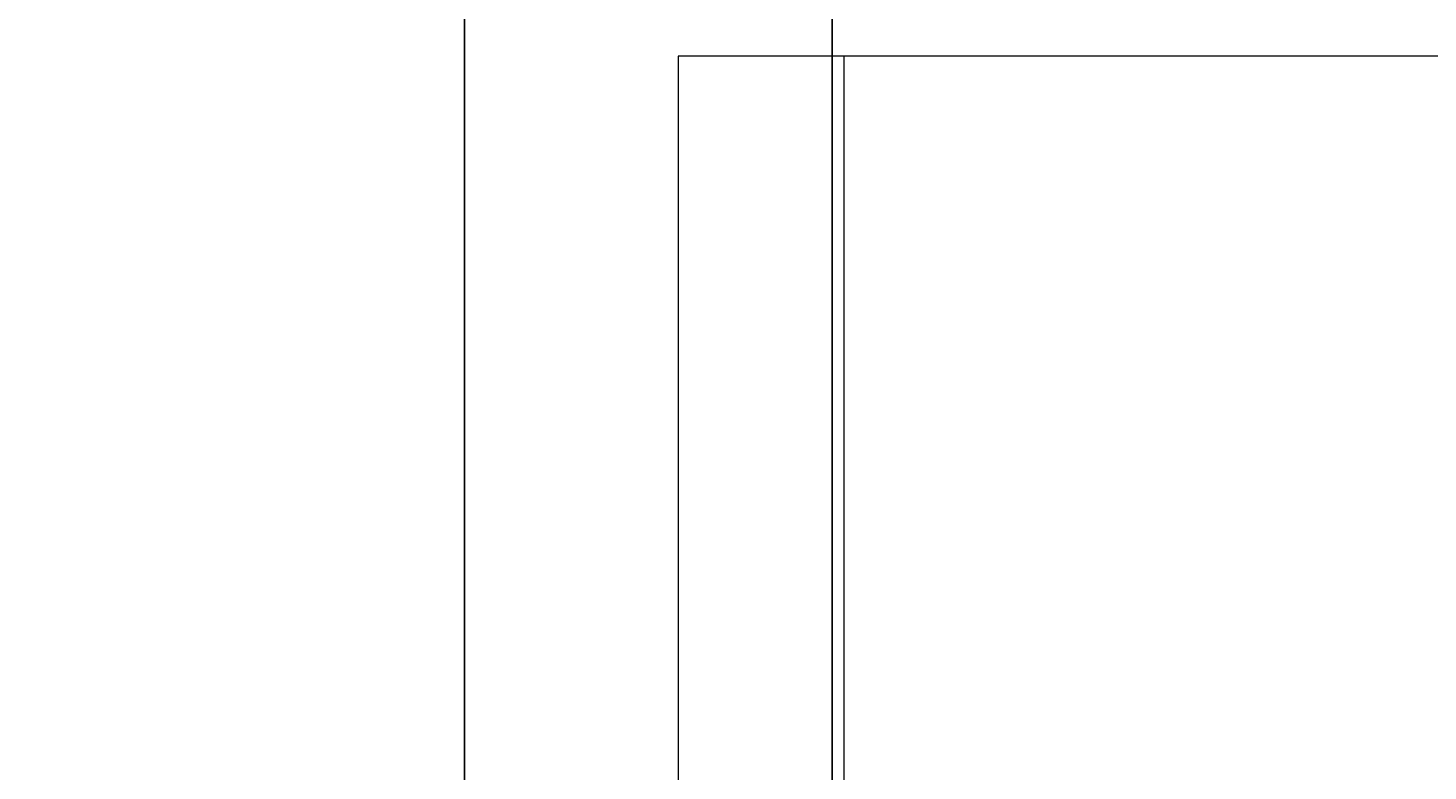
# Model space of a CAD drawing. Units: inches. Extents: x 1998 to 2588, y 1139 to 1977.
# Tile 124 of 134: x 2398 to 2429, y 1653 to 1669. Entities that reach past the tile are written whole.
import ezdxf

# ---------------------------------------------------------------- set-up
doc = ezdxf.new("R2010")
doc.units = ezdxf.units.IN
doc.layers.add('A-ANNO-DIMS', color=2, linetype='Continuous', lineweight=18)
doc.layers.add('FUR', color=21, linetype='Continuous', lineweight=18)
doc.styles.get("Standard").update_dxf_attribs({"font": 'arial.ttf'})
doc.dimstyles.get("Standard").update_dxf_attribs({"dimtxt": 0.18, "dimasz": 0.18, "dimexe": 0.18, "dimexo": 0.0625, "dimgap": 0.09, "dimtad": 0, "dimtih": 1, "dimtoh": 1, "dimdec": 4, "dimzin": 0, "dimdsep": 46, "dimtxsty": 'Standard', "dimcen": 0.09, "dimadec": 0, "dimazin": 0, "dimtfac": 1, "dimtdec": 4, "dimtofl": 0, "dimtmove": 0, "dimatfit": 3, "dimfxl": 1, "dimtolj": 1, "dimtzin": 0, "dimarcsym": 0})

# ---------------------------------------------------------------- blocks, each defined once
blk = doc.blocks.new('SOFA-THREE-SEAT')
for p, q in [((3.604, 25.615), (0, 25.615)), ((0, 25.615), (0, 0))]:
    blk.add_line(p, q)
blk.add_lwpolyline([(3.604, 2.416), (71.008, 2.416), (71.008, 25.615), (3.604, 25.615)], close=True)
blk = doc.blocks.new('*D24')
at = {"layer": 'A-ANNO-DIMS', "color": 0, "lineweight": -2, "transparency": 16777216}
for p, q in [((2398.535, 1911.232), (2588.309, 1911.232)), ((2588.129, 1911.052), (2588.129, 1570.164)), ((2588.129, 1228.912), (2588.129, 1569.8)), ((2527.535, 1228.732), (2588.309, 1228.732))]:
    blk.add_line(p, q, dxfattribs=at)
at = {"layer": 'A-ANNO-DIMS', "color": 0, "transparency": 16777216}
for points in [[(2588.099, 1911.052), (2588.159, 1911.052), (2588.129, 1911.232)], [(2588.099, 1228.912), (2588.159, 1228.912), (2588.129, 1228.732)]]:
    blk.add_solid(points, dxfattribs=at)
at = {"layer": 'Defpoints', "color": 0, "transparency": 16777216}
for p in [(2398.473, 1911.232), (2588.129, 1911.232), (2527.473, 1228.732)]:
    blk.add_point(p, dxfattribs=at)
at = {"layer": 'A-ANNO-DIMS', "color": 0, "transparency": 16777216, "insert": (2588.129, 1569.982), "char_height": 0.18, "attachment_point": 5}
blk.add_mtext('\\A1;682.5', dxfattribs=at)
blk = doc.blocks.new('*D32')
at = {"layer": 'A-ANNO-DIMS', "color": 0, "lineweight": -2, "transparency": 16777216}
for p, q in [((2407.973, 1636.795), (2407.973, 1977.362)), ((2415.973, 1636.795), (2415.973, 1977.362)), ((2408.153, 1977.182), (2411.824, 1977.182)), ((2415.793, 1977.182), (2412.122, 1977.182))]:
    blk.add_line(p, q, dxfattribs=at)
at = {"layer": 'A-ANNO-DIMS', "color": 0, "transparency": 16777216}
for points in [[(2408.153, 1977.212), (2408.153, 1977.152), (2407.973, 1977.182)], [(2415.793, 1977.212), (2415.793, 1977.152), (2415.973, 1977.182)]]:
    blk.add_solid(points, dxfattribs=at)
at = {"layer": 'Defpoints', "color": 0, "transparency": 16777216}
for p in [(2415.973, 1977.182), (2407.973, 1636.732), (2415.973, 1636.732)]:
    blk.add_point(p, dxfattribs=at)
at = {"layer": 'A-ANNO-DIMS', "color": 0, "transparency": 16777216, "insert": (2411.973, 1977.182), "char_height": 0.18, "attachment_point": 5}
blk.add_mtext('\\A1;8', dxfattribs=at)

msp = doc.modelspace()

# ---------------------------------------------------------------- block references
at = {"layer": 'FUR'}
msp.add_blockref('SOFA-THREE-SEAT', (2412.6207, 1642.8172), dxfattribs=at)

# ---------------------------------------------------------------- dimensions: what is measured, and where the dimension line sits
at = {"layer": 'A-ANNO-DIMS'}
dim = msp.add_linear_dim(base=(2415.9729, 1977.1824), p1=(2407.9729, 1636.7324), p2=(2415.9729, 1636.7324), dimstyle='Standard', override={"dimdec": 0, "dimlfac": 1, "dimrnd": 0, "dimzin": 0, "dimdsep": 46, "dimlunit": 2}, dxfattribs=at)
dim.commit()
dim.dimension.update_dxf_attribs({"geometry": '*D32', "text_midpoint": (2411.9729, 1977.1824)})
dim = msp.add_linear_dim(base=(2588.1286, 1911.2324), p1=(2527.4729, 1228.7324), p2=(2398.4729, 1911.2324), angle=90, dimstyle='Standard', override={"dimdec": 1, "dimlfac": 1, "dimrnd": 0, "dimzin": 0, "dimdsep": 46, "dimlunit": 2}, dxfattribs=at)
dim.commit()
dim.dimension.update_dxf_attribs({"geometry": '*D24', "text_midpoint": (2588.1286, 1569.9824)})

doc.saveas('drawing.dxf')
